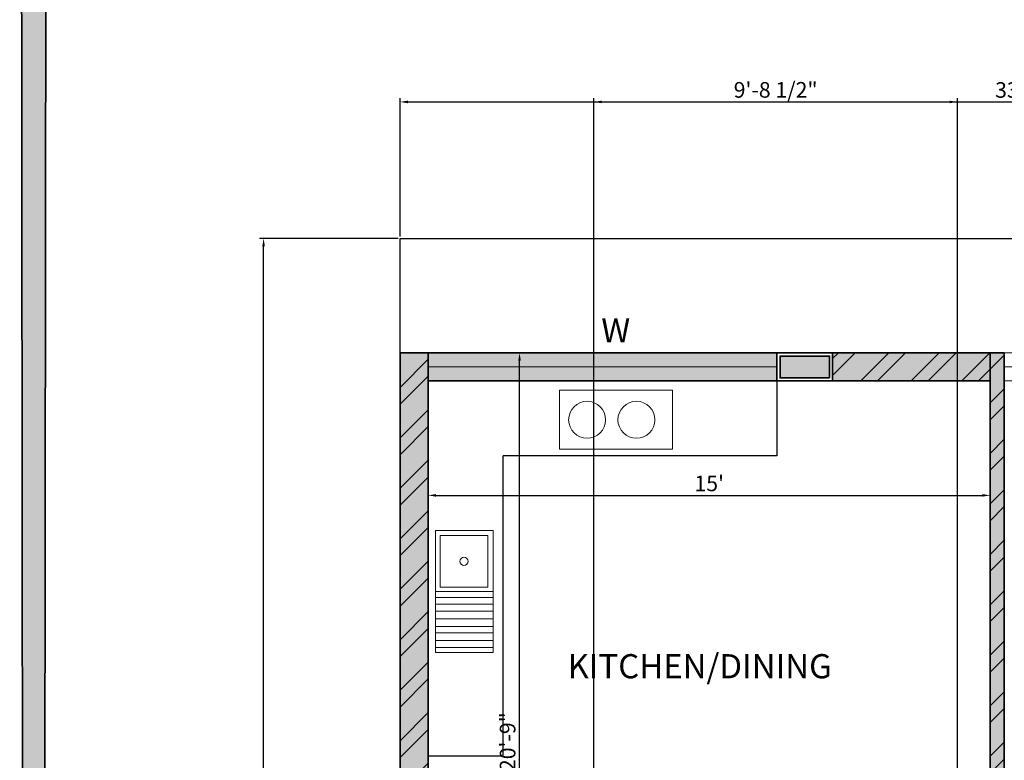
# Model space of a CAD drawing. Units: inches. Extents: x 1804 to 3296, y 909 to 2477.
# Tile 12 of 31: x 1804 to 2119, y 1663 to 1900. Entities that reach past the tile are written whole.
import ezdxf

# ---------------------------------------------------------------- set-up
doc = ezdxf.new("R2010")
doc.units = ezdxf.units.IN
for name, color, linetype, lineweight in [('A-ANNO-DIMS', 2, 'Continuous', 18), ('A-ANNO-TTLB', 156, 'Continuous', 35), ('A-AREA-IDEN', 190, 'Continuous', 18), ('A-EQPM', 9, 'Continuous', 18), ('A-FLOR-CASE', 100, 'Continuous', 25), ('A-FLOR-FIXT', 9, 'Continuous', 18), ('A-WALL-PATT', 10, 'Continuous', 13), ('C-PROP', 7, 'Continuous', 25), ('TEXT', 190, 'Continuous', 18), ('WALL', 10, 'Continuous', 35), ('WIND', 130, 'Continuous', 18)]:
    doc.layers.add(name, color=color, linetype=linetype, lineweight=lineweight)
doc.styles.get("Standard").update_dxf_attribs({"font": 'arial.ttf'})
doc.dimstyles.new('ISO-25', dxfattribs={"dimtxt": 5, "dimasz": 2.5, "dimexe": 1.25, "dimexo": 0.625, "dimtad": 1, "dimdec": 0, "dimlunit": 4, "dimtxsty": 'Standard', "dimcen": 2.5, "dimadec": 0, "dimazin": 0, "dimtfac": 1, "dimtdec": 0, "dimtmove": 0, "dimatfit": 3, "dimfxl": 1, "dimarcsym": 0})
pattern_1 = [(45, (0, 196.207), (-8.08223, 8.08223), []), (45, (5.388, 196.207), (-8.08223, 8.08223), [])]

# ---------------------------------------------------------------- blocks, each defined once
blk = doc.blocks.new('*D8')
at = {"layer": 'A-ANNO-DIMS', "color": 0, "lineweight": -2, "transparency": 16777216}
for p, q in [((1934.58, 1792.75), (1934.58, 1746.51)), ((2114.58, 1792.75), (2114.58, 1746.51)), ((1937.08, 1747.76), (2112.08, 1747.76))]:
    blk.add_line(p, q, dxfattribs=at)
at = {"layer": 'A-ANNO-DIMS', "color": 0, "lineweight": 100, "transparency": 16777216}
for points in [[(1937.08, 1748.17), (1937.08, 1747.34), (1934.58, 1747.76)], [(2112.08, 1748.17), (2112.08, 1747.34), (2114.58, 1747.76)]]:
    blk.add_solid(points, dxfattribs=at)
at = {"layer": 'Defpoints', "color": 0, "lineweight": 100, "transparency": 16777216}
for p in [(1934.58, 1793.38), (2114.58, 1793.38), (2114.58, 1747.76)]:
    blk.add_point(p, dxfattribs=at)
at = {"layer": 'A-ANNO-DIMS', "color": 0, "transparency": 16777216, "insert": (2024.58, 1750.93), "char_height": 5, "attachment_point": 5}
blk.add_mtext("15'", dxfattribs=at)
blk = doc.blocks.new('*D9')
at = {"layer": 'A-ANNO-DIMS', "color": 0, "lineweight": -2, "transparency": 16777216}
for p, q in [((1935.21, 1793.38), (1965.1, 1793.38)), ((1963.85, 1546.88), (1963.85, 1790.88)), ((1935.21, 1544.38), (1965.1, 1544.38))]:
    blk.add_line(p, q, dxfattribs=at)
at = {"layer": 'A-ANNO-DIMS', "color": 0, "lineweight": 100, "transparency": 16777216}
for points in [[(1963.44, 1790.88), (1964.27, 1790.88), (1963.85, 1793.38)], [(1963.44, 1546.88), (1964.27, 1546.88), (1963.85, 1544.38)]]:
    blk.add_solid(points, dxfattribs=at)
at = {"layer": 'Defpoints', "color": 0, "lineweight": 100, "transparency": 16777216}
for p in [(1934.58, 1793.38), (1963.85, 1793.38), (1934.58, 1544.38)]:
    blk.add_point(p, dxfattribs=at)
at = {"layer": 'A-ANNO-DIMS', "color": 0, "transparency": 16777216, "insert": (1960.67, 1668.88), "char_height": 5, "attachment_point": 5, "rotation": 90}
blk.add_mtext('20\'-9"', dxfattribs=at)
blk = doc.blocks.new('WINDOW-PLAN-112IN')
blk.add_line((0, 4.5), (111.7, 4.5))
blk.add_lwpolyline([(0, 0), (111.7, 0), (111.7, 9), (0, 9)], close=True)
blk = doc.blocks.new('*D51')
at = {"layer": 'A-ANNO-DIMS', "color": 0, "lineweight": -2, "transparency": 16777216}
for p, q in [((1925.58, 1830.66), (1925.58, 1874.99)), ((1928.08, 1873.74), (2323.04, 1873.74)), ((2325.54, 1830.66), (2325.54, 1874.99))]:
    blk.add_line(p, q, dxfattribs=at)
at = {"layer": 'A-ANNO-DIMS', "color": 0, "lineweight": 100, "transparency": 16777216}
for points in [[(1928.08, 1874.15), (1928.08, 1873.32), (1925.58, 1873.74)], [(2323.04, 1874.15), (2323.04, 1873.32), (2325.54, 1873.74)]]:
    blk.add_solid(points, dxfattribs=at)
at = {"layer": 'Defpoints', "color": 0, "lineweight": 100, "transparency": 16777216}
for p in [(2325.54, 1873.74), (1925.58, 1830.04), (2325.54, 1830.04)]:
    blk.add_point(p, dxfattribs=at)
at = {"layer": 'A-ANNO-DIMS', "color": 0, "transparency": 16777216, "insert": (2125.56, 1876.92), "char_height": 5, "attachment_point": 5}
blk.add_mtext('33\'-4"', dxfattribs=at)
blk = doc.blocks.new('*D52')
at = {"layer": 'A-ANNO-DIMS', "color": 0, "lineweight": -2, "transparency": 16777216}
for p, q in [((1924.96, 1830.04), (1880.63, 1830.04)), ((1881.88, 1065.27), (1881.88, 1827.54)), ((1924.96, 1062.77), (1880.63, 1062.77))]:
    blk.add_line(p, q, dxfattribs=at)
at = {"layer": 'A-ANNO-DIMS', "color": 0, "lineweight": 100, "transparency": 16777216}
for points in [[(1881.47, 1827.54), (1882.3, 1827.54), (1881.88, 1830.04)], [(1881.47, 1065.27), (1882.3, 1065.27), (1881.88, 1062.77)]]:
    blk.add_solid(points, dxfattribs=at)
at = {"layer": 'Defpoints', "color": 0, "lineweight": 100, "transparency": 16777216}
for p in [(1881.88, 1830.04), (1925.58, 1830.04), (1925.58, 1062.77)]:
    blk.add_point(p, dxfattribs=at)
at = {"layer": 'A-ANNO-DIMS', "color": 0, "transparency": 16777216, "insert": (1878.67, 1446.4), "char_height": 5, "attachment_point": 5, "rotation": 90}
blk.add_mtext('63\'-11 1/2"', dxfattribs=at)
blk = doc.blocks.new('*D62')
at = {"layer": 'A-ANNO-DIMS', "color": 0, "lineweight": -2, "transparency": 16777216}
for p, q in [((1987.63, 1501.57), (1987.63, 1874.99)), ((1990.13, 1873.74), (2101.57, 1873.74)), ((2104.07, 1501.57), (2104.07, 1874.99))]:
    blk.add_line(p, q, dxfattribs=at)
at = {"layer": 'A-ANNO-DIMS', "color": 0, "lineweight": 100, "transparency": 16777216}
for points in [[(1990.13, 1874.15), (1990.13, 1873.32), (1987.63, 1873.74)], [(2101.57, 1874.15), (2101.57, 1873.32), (2104.07, 1873.74)]]:
    blk.add_solid(points, dxfattribs=at)
at = {"layer": 'Defpoints', "color": 0, "lineweight": 100, "transparency": 16777216}
for p in [(2104.07, 1873.74), (1987.63, 1500.95), (2104.07, 1500.95)]:
    blk.add_point(p, dxfattribs=at)
at = {"layer": 'A-ANNO-DIMS', "color": 0, "transparency": 16777216, "insert": (2045.85, 1876.95), "char_height": 5, "attachment_point": 5}
blk.add_mtext('9\'-8 1/2"', dxfattribs=at)

msp = doc.modelspace()

# ---------------------------------------------------------------- hatches: boundary and pattern name
at = {"layer": 'A-ANNO-TTLB'}
h = msp.add_hatch(color=256, dxfattribs=at)
h.dxf.hatch_style = 1
h.paths.add_polyline_path([(3294.53, 2476.54), (1803.79, 2476.54), (1805.43, 909.47), (3296.17, 909.47)])
h.paths.add_polyline_path([(1811, 914.33), (1812.79, 2467.54), (3285.53, 2467.54), (3283.74, 914.33)], flags=16)
h.paths.add_polyline_path([(1925.58, 1062.77), (1925.58, 1138.07), (1925.58, 1539.88), (1925.58, 1793.38), (1925.58, 1830.04), (2325.54, 1830.04), (2325.54, 1793.38), (2325.54, 1586.42), (2325.54, 1138.07), (2325.54, 1062.77)], flags=0)
h.paths.add_polyline_path([(1997.22, 1029.4), (2008.85, 1037.96), (2008.85, 1020.84)], flags=0)
h.paths.add_polyline_path([(1934.58, 1138.07), (1934.58, 1147.07), (2078.77, 1147.07), (2078.77, 1138.07), (2060.94, 1138.07)], flags=0)
h.paths.add_polyline_path([(1944.35, 1138.07), (1944.35, 1147.07), (2056.05, 1147.07), (2056.05, 1138.07)], flags=0)
h.paths.add_polyline_path([(2222.24, 1037.96), (2233.87, 1029.4), (2222.24, 1020.84)], flags=0)
h.paths.add_polyline_path([(2061.94, 1139.07), (2061.94, 1146.07), (2077.77, 1146.07), (2077.77, 1139.07)], flags=0)
h.paths.add_polyline_path([(2149.58, 1138.07), (2149.58, 1269.44), (2158.58, 1269.44), (2158.58, 1326.69), (2149.58, 1326.69), (2149.58, 1340.94), (2139.6, 1340.94), (2139.6, 1434.25), (2149.58, 1434.25), (2149.58, 1447.36), (2158.58, 1447.36), (2158.58, 1423.87), (2158.58, 1408.06), (2198.46, 1408.06), (2198.46, 1412.56), (2282.65, 1412.56), (2282.65, 1465.94), (2316.54, 1465.94), (2316.54, 1590.92), (2192.86, 1590.92), (2192.86, 1595.3), (2291.17, 1595.3), (2291.17, 1590.92), (2316.54, 1590.92), (2316.54, 1784.38), (2300.24, 1784.38), (2300.24, 1757.47), (2268, 1757.47), (2268, 1681.04), (2180.87, 1681.04), (2180.87, 1757.47), (2148.63, 1757.47), (2148.63, 1784.38), (2119.08, 1784.38), (2119.08, 1585.58), (2114.58, 1585.58), (2114.58, 1784.38), (2064.11, 1784.38), (2046.28, 1784.38), (2046.28, 1760.38), (1958.58, 1760.38), (1958.58, 1664.38), (1934.58, 1664.38), (1934.58, 1784.38), (1934.58, 1793.38), (2046.28, 1793.38), (2064.11, 1793.38), (2119.08, 1793.38), (2230.78, 1793.38), (2230.78, 1784.38), (2268, 1784.38), (2300.24, 1784.38), (2316.54, 1784.38), (2316.54, 1590.92), (2316.54, 1373.73), (2316.54, 1138.07)], flags=0)
h.paths.add_polyline_path([(2209.19, 1166.63), (2209.19, 1175.63), (2158.58, 1175.63), (2209.19, 1223.63), (2209.19, 1231.63), (2183.88, 1231.63), (2183.88, 1301.66), (2242.59, 1301.66), (2242.59, 1326.69), (2316.54, 1326.69), (2272.59, 1271.63), (2272.59, 1223.63), (2316.54, 1175.63), (2272.59, 1175.63), (2272.59, 1166.63)], flags=0)
h.paths.add_polyline_path([(1947.77, 1345.22), (1947.77, 1457.48), (1991.2, 1457.48), (1991.2, 1451.7), (1991.2, 1352.18), (1991.2, 1345.22)], flags=0)
h.paths.add_polyline_path([(2209.19, 1271.63), (2262.59, 1271.63), (2262.59, 1311.85), (2272.59, 1301.66), (2272.59, 1271.63), (2269.92, 1269.63), (2270.59, 1269.63), (2270.59, 1225.63), (2211.19, 1225.63), (2211.19, 1269.63), (2211.86, 1269.63)], flags=0)
h.paths.add_polyline_path([(2000.34, 1378.21), (2000.34, 1429.71), (2025.22, 1429.71), (2025.22, 1378.21)], flags=0)
h.paths.add_polyline_path([(2001.34, 1379.21), (2001.34, 1428.71), (2024.22, 1428.71), (2024.22, 1379.21)], flags=0)
h.paths.add_polyline_path([(2012.34, 1390.21), (2012.34, 1417.71), (2013.22, 1417.71), (2013.22, 1390.21)], flags=0)
h.paths.add_polyline_path([(2237.56, 1331.19), (2237.56, 1340.18), (2238.62, 1340.18), (2238.62, 1386.84), (2241.04, 1386.84), (2242.06, 1386.84), (2242.06, 1408.06), (2316.54, 1331.19)], flags=0)
h.paths.add_polyline_path([(1953.73, 1464.35), (1953.73, 1498.59), (1981.74, 1498.59), (1981.74, 1464.35)], flags=0)
h.paths.add_polyline_path([(1987.63, 1462.08), (1987.63, 1500.95), (2104.07, 1500.95), (2104.07, 1462.08), (2099.27, 1462.08), (1993.6, 1462.08)], flags=0)
h.paths.add_polyline_path([(1956.06, 1481.47, -1), (1979.41, 1481.47, -1)], flags=0)
edge = h.paths.add_edge_path(flags=0)
edge.add_ellipse((2299.53, 1438.37), major_axis=(0.31, 21.36), ratio=0.670333, start_angle=0, end_angle=360)
h.paths.add_polyline_path([(2297.39, 1438.37, -1), (2301.67, 1438.37, -1)], flags=0)
h.paths.add_polyline_path([(2591.54, 1163.23), (2591.54, 1179.38), (2591.54, 1379.68), (2591.54, 1395.84), (2734.5, 1395.84), (2734.5, 1379.68), (2734.5, 1179.38), (2734.5, 1163.23)], flags=0)
h.paths.add_polyline_path([(2592.54, 1164.23), (2592.54, 1166.23), (2733.5, 1166.23), (2733.5, 1164.23)], flags=0)
h.paths.add_polyline_path([(2592.54, 1180.38), (2592.54, 1378.68), (2733.5, 1378.68), (2733.5, 1180.38)], flags=0)
h.paths.add_polyline_path([(2593.54, 1181.38), (2593.54, 1377.68), (2732.5, 1377.68), (2732.5, 1181.38)], flags=0)
h.paths.add_polyline_path([(2594.54, 1182.38), (2594.54, 1376.68), (2731.5, 1376.68), (2731.5, 1182.38)], flags=0)
h.paths.add_polyline_path([(1936.95, 1697.46), (1936.95, 1736.46), (1955.41, 1736.46), (1955.41, 1697.46)], flags=0)
h.paths.add_polyline_path([(1938.48, 1718.36), (1938.48, 1734.92), (1953.65, 1734.92), (1953.65, 1718.36)], flags=0)
h.paths.add_polyline_path([(1944.75, 1726.64, -1), (1947.37, 1726.64, -1)], flags=0)
h.paths.add_polyline_path([(2592.54, 1394.84), (2733.5, 1394.84), (2733.5, 1392.84), (2592.54, 1392.84)], flags=0)
h.paths.add_polyline_path([(1976.61, 1762.5), (1976.61, 1781.44), (2012.79, 1781.44), (2012.79, 1762.5)], flags=0)
h.paths.add_polyline_path([(1979.57, 1771.97, -1), (1991.39, 1771.97, -1)], flags=0)
h.paths.add_polyline_path([(1995.36, 1771.97, -1), (2007.18, 1771.97, -1)], flags=0)
h.paths.add_polyline_path([(2251.51, 1744.53), (2268, 1730.05), (2251.51, 1730.05)], flags=0)
h.paths.add_polyline_path([(2047.28, 1785.38), (2047.28, 1792.38), (2063.11, 1792.38), (2063.11, 1785.38)], flags=0)
h.paths.add_polyline_path([(2155.08, 1770.92, -1), (2174.42, 1770.92, -1)], flags=0)
h.paths.add_polyline_path([(2188.59, 1758.27), (2188.59, 1772.81), (2222.3, 1772.81), (2222.3, 1758.27)], flags=0)
h.paths.add_polyline_path([(2223.97, 1758.27), (2223.97, 1772.81), (2257.68, 1772.81), (2257.68, 1758.27)], flags=0)
h.paths.add_polyline_path([(2274.45, 1770.92, -1), (2293.8, 1770.92, -1)], flags=0)
h.paths.add_polyline_path([(2591.54, 1582.09), (2591.54, 1782.39), (2734.5, 1782.39), (2734.5, 1582.09)], flags=0)
h.paths.add_polyline_path([(2592.54, 1583.09), (2592.54, 1781.39), (2733.5, 1781.39), (2733.5, 1583.09)], flags=0)
h.paths.add_polyline_path([(2593.54, 1584.09), (2593.54, 1780.39), (2732.5, 1780.39), (2732.5, 1584.09)], flags=0)
h.paths.add_polyline_path([(2594.54, 1585.09), (2594.54, 1779.39), (2731.5, 1779.39), (2731.5, 1585.09)], flags=0)
h.paths.add_polyline_path([(1922.17, 1978.79), (1922.17, 2295.08), (1922.17, 2296.08), (2115.67, 2296.08), (2115.67, 2384.31), (2115.67, 2385.31), (2322.12, 2385.31), (2323.12, 2385.31), (2323.12, 1979.79), (2323.12, 1978.79), (1923.17, 1978.79)], flags=0)
h.paths.add_polyline_path([(1922.17, 1978.79), (1922.17, 2051.31), (1922.17, 2214.86), (1922.17, 2296.08), (2115.67, 2296.08), (2115.67, 2385.31), (2323.12, 2385.31), (2323.12, 2280.42), (2323.12, 1978.79), (2115.67, 1978.79)], flags=0)
h.paths.add_polyline_path([(1923.17, 1979.79), (1923.17, 2050.31), (2115.67, 2050.31), (2115.67, 2051.31), (1923.17, 2051.31), (1923.17, 2213.86), (1923.17, 2214.86), (1923.17, 2295.08), (1990.02, 2295.08), (1990.02, 2214.86), (1991.02, 2214.86), (1991.02, 2295.08), (2115.67, 2295.08), (2115.67, 1979.79), (2116.67, 1979.79), (2116.67, 2304.18), (2116.67, 2384.31), (2322.12, 2384.31), (2322.12, 2280.42), (2322.12, 1979.79), (2115.67, 1979.79)], flags=0)
h.paths.add_polyline_path([(2972.46, 1192.5), (2972.46, 1196.92), (2995.47, 1196.92), (2995.47, 1255.47), (2995.09, 1255.47), (2987.42, 1249.39), (2980.08, 1255.47), (2978.05, 1255.47), (2978.05, 1257.24), (2995.47, 1257.24), (2995.47, 1261.58), (3015.37, 1261.58), (3015.37, 1333.28), (3015.37, 1414.4), (3032.82, 1414.4), (3032.82, 1333.28), (3032.82, 1261.58), (3052.66, 1261.58), (3052.66, 1255.47), (3079.86, 1255.47), (3078.72, 1254.57), (3081.47, 1252.29), (3078.56, 1249.99), (3075.81, 1252.26), (3072.57, 1249.69), (3070.36, 1251.52), (3067.67, 1249.39), (3060.34, 1255.47), (3052.66, 1255.47), (3052.66, 1196.92), (3054.58, 1196.92), (3074, 1196.92), (3074, 1192.5), (3052.66, 1192.5), (2995.47, 1192.5)], flags=0)
h.paths.add_polyline_path([(2490.75, 1979.27), (2490.75, 1980.27), (2596.87, 1980.27), (2596.87, 2051.8), (2596.87, 2052.8), (2596.87, 2216.35), (2596.87, 2297.57), (2717.32, 2297.57), (2710.57, 2305.62), (2724.07, 2305.62), (2717.32, 2297.57), (2782.37, 2297.57), (2782.37, 2395.8), (3006.82, 2395.8), (3006.82, 1981.27), (3093.73, 1981.27), (3093.73, 1980.27), (3047.51, 1980.27), (3046.37, 1979.37), (3049.11, 1977.1), (3046.2, 1974.79), (3043.46, 1977.07), (3040.21, 1974.49), (3038, 1976.32), (3035.32, 1974.2), (3027.98, 1980.27), (2871.83, 1980.27), (2871.83, 1981.27), (2791.37, 1981.27), (2791.37, 2050.8), (2597.87, 2050.8), (2597.87, 1980.27), (2597.87, 1979.27), (2546.27, 1979.27), (2545.12, 1978.37), (2547.87, 1976.1), (2544.96, 1973.79), (2542.22, 1976.07), (2538.97, 1973.49), (2536.76, 1975.32), (2534.07, 1973.2), (2526.74, 1979.27)], flags=0)
h.paths.add_polyline_path([(2597.87, 2051.8), (2606.87, 2051.8), (2606.87, 2258.39), (2597.87, 2258.39), (2597.87, 2296.57), (2606.87, 2296.57), (2606.87, 2262.39), (2782.37, 2262.39), (2782.37, 2296.57), (2790.37, 2296.57), (2790.37, 2262.39), (2791.37, 2262.39), (2791.37, 2305.67), (2791.37, 2385.8), (2996.82, 2385.8), (2996.82, 2339.85), (3006.82, 2339.85), (3006.82, 2250.12), (2997.82, 2250.12), (2997.82, 1981.27), (2996.82, 1981.27), (2872.83, 1981.27), (2872.83, 1991.8), (2871.83, 1991.8), (2871.83, 2050.8), (2790.37, 2050.8), (2597.87, 2050.8)], flags=0)
h.paths.add_polyline_path([(2179.93, 2153.92), (2179.93, 2353.97), (2259.98, 2353.97), (2259.98, 2153.92)], flags=0)
h.paths.add_polyline_path([(2180.93, 2154.92), (2180.93, 2352.97), (2258.98, 2352.97), (2258.98, 2154.92)], flags=0)
h.paths.add_polyline_path([(2960.87, 1608.49), (2960.87, 1753.62), (3070.9, 1753.62), (3070.9, 1608.49)], flags=0)
h.paths.add_polyline_path([(2961.87, 1609.49), (2961.87, 1752.62), (3069.9, 1752.62), (3069.9, 1609.49)], flags=0)
h.paths.add_polyline_path([(2962.87, 1610.49), (2962.87, 1751.62), (3068.9, 1751.62), (3068.9, 1610.49)], flags=0)
h.paths.add_polyline_path([(2963.87, 1611.49), (2963.87, 1750.62), (3067.9, 1750.62), (3067.9, 1611.49)], flags=0)
h.paths.add_polyline_path([(2782.37, 2051.8), (2782.37, 2216.32), (2791.37, 2216.32), (2791.37, 2051.8), (2872.83, 2051.8), (2872.83, 2068.56), (2884.67, 2068.56), (2884.67, 2085.33), (2896.51, 2085.33), (2896.51, 2102.09), (2908.36, 2102.09), (2908.36, 2118.85), (2920.2, 2118.85), (2920.2, 2135.62), (2932.05, 2135.62), (2932.05, 2145.3), (2925.08, 2145.3), (2925.08, 2203.2), (2996.82, 2203.2), (2996.82, 2145.3), (2953.82, 2145.3), (2872.83, 2051.8), (2790.37, 2051.8)], flags=0)
h.paths.add_polyline_path([(2717.32, 2238.65), (2710.57, 2246.7), (2724.07, 2246.7)], flags=0)
h.paths.add_polyline_path([(2003.09, 1122.79), (2017.16, 1122.79), (2017.16, 1138.74), (2003.09, 1138.74)], flags=8)
h.paths.add_polyline_path([(2174.76, 1792.72), (2188.83, 1792.72), (2188.83, 1808.66), (2174.76, 1808.66)], flags=8)
h.paths.add_polyline_path([(1987.95, 1792.51), (2002.02, 1792.51), (2002.02, 1808.45), (1987.95, 1808.45)], flags=8)
h.paths.add_polyline_path([(2148.79, 1289.26), (2160.46, 1289.26), (2160.46, 1305.2), (2148.79, 1305.2)], flags=8)
h.paths.add_polyline_path([(2115.36, 1133.57), (2127.04, 1133.57), (2127.04, 1149.51), (2115.36, 1149.51)], flags=8)
h.paths.add_polyline_path([(2237.58, 1421.48), (2249.25, 1421.48), (2249.25, 1437.43), (2237.58, 1437.43)], flags=8)
h.paths.add_polyline_path([(2134.99, 1584.32), (2146.66, 1584.32), (2146.66, 1600.26), (2134.99, 1600.26)], flags=8)
h.paths.add_polyline_path([(2101.95, 1557.31), (2113.62, 1557.31), (2113.62, 1573.25), (2101.95, 1573.25)], flags=8)
h.paths.add_polyline_path([(2937.85, 1156.77), (3120.41, 1156.77), (3120.41, 1185.72), (2937.85, 1185.72)], flags=8)
h.paths.add_polyline_path([(2980.71, 1786.71), (3050.06, 1786.71), (3050.06, 1802.66), (2980.71, 1802.66)], flags=8)
h.paths.add_polyline_path([(2869.28, 1661.96), (2938.62, 1661.96), (2938.62, 1690.8), (2869.28, 1690.8)], flags=8)
h.paths.add_polyline_path([(3092.27, 1674.86), (3161.62, 1674.86), (3161.62, 1690.8), (3092.27, 1690.8)], flags=8)
h.paths.add_polyline_path([(2980.71, 1674.86), (3050.06, 1674.86), (3050.06, 1690.8), (2980.71, 1690.8)], flags=8)
h.paths.add_polyline_path([(2649.07, 1678.23), (2674.53, 1678.23), (2674.53, 1714.76), (2649.07, 1714.76)], flags=8)
h.paths.add_polyline_path([(2530.84, 1981.63), (2549.13, 1981.63), (2549.13, 1997.57), (2530.84, 1997.57)], flags=8)
h.paths.add_polyline_path([(3031.29, 1981.77), (3049.58, 1981.77), (3049.58, 1997.71), (3031.29, 1997.71)], flags=8)
h.paths.add_polyline_path([(2715.38, 1911.9), (2851.54, 1911.9), (2851.54, 1940.85), (2715.38, 1940.85)], flags=8)
h.paths.add_polyline_path([(2015.23, 1927.36), (2205.42, 1927.36), (2205.42, 1956.3), (2015.23, 1956.3)], flags=8)
h.paths.add_polyline_path([(2671.84, 2057.84), (2702.75, 2057.84), (2702.75, 2073.79), (2671.84, 2073.79)], flags=8)
h.paths.add_polyline_path([(2678.5, 2316.52), (2765.26, 2316.52), (2765.26, 2332.46), (2678.5, 2332.46)], flags=8)
h.paths.add_polyline_path([(2678.48, 2271.96), (2736.41, 2271.96), (2736.41, 2287.9), (2678.48, 2287.9)], flags=8)
h.paths.add_polyline_path([(2019.2, 972.79), (2243.21, 972.79), (2243.21, 1001.74), (2019.2, 1001.74)], flags=8)
h.paths.add_polyline_path([(2097.06, 1021.56), (2132.16, 1021.56), (2132.16, 1037.51), (2097.06, 1037.51)], flags=8)
h.paths.add_polyline_path([(2182.47, 1360.48), (2207.35, 1360.48), (2207.35, 1376.42), (2182.47, 1376.42)], flags=8)
h.paths.add_polyline_path([(2261.12, 1361.77), (2295.01, 1361.77), (2295.01, 1377.71), (2261.12, 1377.71)], flags=8)
h.paths.add_polyline_path([(2245.75, 1511.51), (2278.44, 1511.51), (2278.44, 1527.46), (2245.75, 1527.46)], flags=8)
h.paths.add_polyline_path([(1991.16, 1296.29), (2060.51, 1296.29), (2060.51, 1312.23), (1991.16, 1312.23)], flags=8)
h.paths.add_polyline_path([(2187, 1651.35), (2246.71, 1651.35), (2246.71, 1667.29), (2187, 1667.29)], flags=8)
h.paths.add_polyline_path([(1976.49, 1684.81), (2068.63, 1684.81), (2068.63, 1700.76), (1976.49, 1700.76)], flags=8)
at = {"layer": 'A-WALL-PATT'}
h = msp.add_hatch(color=256, dxfattribs=at)
h.dxf.hatch_style = 1
h.paths.add_polyline_path([(2119.08, 1544.38), (1925.58, 1544.38), (1925.58, 1539.88), (2119.08, 1539.88)])
h.paths.add_polyline_path([(2119.08, 1545.58), (2114.58, 1545.58), (2114.58, 1544.38), (2119.08, 1544.38)])
h.paths.add_polyline_path([(1965.87, 1658.79), (1965.87, 1679.09), (1955.57, 1679.09), (1955.57, 1658.79)], flags=9)
h.paths.add_polyline_path([(2293.18, 1677.29), (2293.18, 1697.58), (2282.88, 1697.58), (2282.88, 1677.29)], flags=9)
h.paths.add_polyline_path([(2271.13, 1545.23), (2287.53, 1545.23), (2287.53, 1555.53), (2271.13, 1555.53)], flags=9)
h.paths.add_polyline_path([(2303.26, 1488.52), (2303.26, 1508.82), (2292.95, 1508.82), (2292.95, 1488.52)], flags=9)
h.paths.add_polyline_path([(2271.13, 1393.15), (2287.53, 1393.15), (2287.53, 1403.45), (2271.13, 1403.45)], flags=9)
h.paths.add_polyline_path([(2306.48, 1361.45), (2306.48, 1377.86), (2296.18, 1377.86), (2296.18, 1361.45)], flags=9)
h.paths.add_polyline_path([(2174.54, 1361.45), (2174.54, 1377.86), (2164.23, 1377.86), (2164.23, 1361.45)], flags=9)
h.paths.add_polyline_path([(1968.21, 1333.34), (1968.21, 1353.64), (1957.91, 1353.64), (1957.91, 1333.34)], flags=9)
h.paths.add_polyline_path([(2003.09, 1122.79), (2017.16, 1122.79), (2017.16, 1138.74), (2003.09, 1138.74)], flags=9)
h.paths.add_polyline_path([(2174.76, 1792.72), (2188.83, 1792.72), (2188.83, 1808.66), (2174.76, 1808.66)], flags=9)
h.paths.add_polyline_path([(1987.95, 1792.51), (2002.02, 1792.51), (2002.02, 1808.45), (1987.95, 1808.45)], flags=9)
h.paths.add_polyline_path([(2148.79, 1289.26), (2160.46, 1289.26), (2160.46, 1305.2), (2148.79, 1305.2)], flags=9)
h.paths.add_polyline_path([(2115.36, 1133.57), (2127.04, 1133.57), (2127.04, 1149.51), (2115.36, 1149.51)], flags=9)
h.paths.add_polyline_path([(2237.58, 1421.48), (2249.25, 1421.48), (2249.25, 1437.43), (2237.58, 1437.43)], flags=9)
h.paths.add_polyline_path([(2134.99, 1584.32), (2146.66, 1584.32), (2146.66, 1600.26), (2134.99, 1600.26)], flags=9)
h.paths.add_polyline_path([(2101.95, 1557.31), (2113.62, 1557.31), (2113.62, 1573.25), (2101.95, 1573.25)], flags=9)
h.paths.add_polyline_path([(2937.85, 1156.77), (3120.41, 1156.77), (3120.41, 1185.72), (2937.85, 1185.72)], flags=9)
h.paths.add_polyline_path([(2980.71, 1786.71), (3050.06, 1786.71), (3050.06, 1802.66), (2980.71, 1802.66)], flags=9)
h.paths.add_polyline_path([(2869.28, 1661.96), (2938.62, 1661.96), (2938.62, 1690.8), (2869.28, 1690.8)], flags=9)
h.paths.add_polyline_path([(3092.27, 1674.86), (3161.62, 1674.86), (3161.62, 1690.8), (3092.27, 1690.8)], flags=9)
h.paths.add_polyline_path([(2980.71, 1674.86), (3050.06, 1674.86), (3050.06, 1690.8), (2980.71, 1690.8)], flags=9)
h.paths.add_polyline_path([(2649.07, 1678.23), (2674.53, 1678.23), (2674.53, 1714.76), (2649.07, 1714.76)], flags=9)
h.paths.add_polyline_path([(2530.84, 1981.63), (2549.13, 1981.63), (2549.13, 1997.57), (2530.84, 1997.57)], flags=9)
h.paths.add_polyline_path([(3031.29, 1981.77), (3049.58, 1981.77), (3049.58, 1997.71), (3031.29, 1997.71)], flags=9)
h.paths.add_polyline_path([(2715.38, 1911.9), (2851.54, 1911.9), (2851.54, 1940.85), (2715.38, 1940.85)], flags=9)
h.paths.add_polyline_path([(2015.23, 1927.36), (2205.42, 1927.36), (2205.42, 1956.3), (2015.23, 1956.3)], flags=9)
h.paths.add_polyline_path([(2671.84, 2057.84), (2702.75, 2057.84), (2702.75, 2073.79), (2671.84, 2073.79)], flags=9)
h.paths.add_polyline_path([(2678.5, 2316.52), (2765.26, 2316.52), (2765.26, 2332.46), (2678.5, 2332.46)], flags=9)
h.paths.add_polyline_path([(2678.48, 2271.96), (2736.41, 2271.96), (2736.41, 2287.9), (2678.48, 2287.9)], flags=9)
h.paths.add_polyline_path([(2019.2, 972.79), (2243.21, 972.79), (2243.21, 1001.74), (2019.2, 1001.74)], flags=9)
h.paths.add_polyline_path([(2097.06, 1021.56), (2132.16, 1021.56), (2132.16, 1037.51), (2097.06, 1037.51)], flags=9)
h.paths.add_polyline_path([(2182.47, 1360.48), (2207.35, 1360.48), (2207.35, 1376.42), (2182.47, 1376.42)], flags=9)
h.paths.add_polyline_path([(2261.12, 1361.77), (2295.01, 1361.77), (2295.01, 1377.71), (2261.12, 1377.71)], flags=9)
h.paths.add_polyline_path([(2245.75, 1511.51), (2278.44, 1511.51), (2278.44, 1527.46), (2245.75, 1527.46)], flags=9)
h.paths.add_polyline_path([(1991.16, 1296.29), (2060.51, 1296.29), (2060.51, 1312.23), (1991.16, 1312.23)], flags=9)
h.paths.add_polyline_path([(2187, 1651.35), (2246.71, 1651.35), (2246.71, 1667.29), (2187, 1667.29)], flags=9)
h.paths.add_polyline_path([(1976.49, 1684.81), (2068.63, 1684.81), (2068.63, 1700.76), (1976.49, 1700.76)], flags=9)
h = msp.add_hatch(color=256, dxfattribs=at)
h.dxf.hatch_style = 1
h.paths.add_polyline_path([(2149.58, 1147.07), (2141.21, 1147.07), (2141.21, 1144.07), (2141.21, 1138.07), (2149.58, 1138.07)])
h.paths.add_polyline_path([(2101.21, 1144.07, -0.01877), (2101.32, 1147.07), (2078.77, 1147.07), (2078.77, 1138.07), (2101.21, 1138.07)])
h.paths.add_polyline_path([(2060.94, 1147.07), (2056.05, 1147.07), (2056.05, 1138.07), (2060.94, 1138.07)])
h.paths.add_polyline_path([(1944.35, 1147.07), (1934.58, 1147.07), (1934.58, 1138.07), (1944.35, 1138.07)])
h.paths.add_polyline_path([(2158.58, 1269.44), (2149.58, 1269.44), (2149.58, 1138.07), (2158.58, 1138.07)])
h.paths.add_polyline_path([(2003.09, 1122.79), (2017.16, 1122.79), (2017.16, 1138.74), (2003.09, 1138.74)], flags=9)
h.paths.add_polyline_path([(2174.76, 1792.72), (2188.83, 1792.72), (2188.83, 1808.66), (2174.76, 1808.66)], flags=9)
h.paths.add_polyline_path([(1987.95, 1792.51), (2002.02, 1792.51), (2002.02, 1808.45), (1987.95, 1808.45)], flags=9)
h.paths.add_polyline_path([(2148.79, 1289.26), (2160.46, 1289.26), (2160.46, 1305.2), (2148.79, 1305.2)], flags=9)
h.paths.add_polyline_path([(2115.36, 1133.57), (2127.04, 1133.57), (2127.04, 1149.51), (2115.36, 1149.51)], flags=9)
h.paths.add_polyline_path([(2237.58, 1421.48), (2249.25, 1421.48), (2249.25, 1437.43), (2237.58, 1437.43)], flags=9)
h.paths.add_polyline_path([(2134.99, 1584.32), (2146.66, 1584.32), (2146.66, 1600.26), (2134.99, 1600.26)], flags=9)
h.paths.add_polyline_path([(2101.95, 1557.31), (2113.62, 1557.31), (2113.62, 1573.25), (2101.95, 1573.25)], flags=9)
h.paths.add_polyline_path([(2937.85, 1156.77), (3120.41, 1156.77), (3120.41, 1185.72), (2937.85, 1185.72)], flags=9)
h.paths.add_polyline_path([(2980.71, 1786.71), (3050.06, 1786.71), (3050.06, 1802.66), (2980.71, 1802.66)], flags=9)
h.paths.add_polyline_path([(2869.28, 1661.96), (2938.62, 1661.96), (2938.62, 1690.8), (2869.28, 1690.8)], flags=9)
h.paths.add_polyline_path([(3092.27, 1674.86), (3161.62, 1674.86), (3161.62, 1690.8), (3092.27, 1690.8)], flags=9)
h.paths.add_polyline_path([(2980.71, 1674.86), (3050.06, 1674.86), (3050.06, 1690.8), (2980.71, 1690.8)], flags=9)
h.paths.add_polyline_path([(2649.07, 1678.23), (2674.53, 1678.23), (2674.53, 1714.76), (2649.07, 1714.76)], flags=9)
h.paths.add_polyline_path([(2530.84, 1981.63), (2549.13, 1981.63), (2549.13, 1997.57), (2530.84, 1997.57)], flags=9)
h.paths.add_polyline_path([(3031.29, 1981.77), (3049.58, 1981.77), (3049.58, 1997.71), (3031.29, 1997.71)], flags=9)
h.paths.add_polyline_path([(2715.38, 1911.9), (2851.54, 1911.9), (2851.54, 1940.85), (2715.38, 1940.85)], flags=9)
h.paths.add_polyline_path([(2015.23, 1927.36), (2205.42, 1927.36), (2205.42, 1956.3), (2015.23, 1956.3)], flags=9)
h.paths.add_polyline_path([(2671.84, 2057.84), (2702.75, 2057.84), (2702.75, 2073.79), (2671.84, 2073.79)], flags=9)
h.paths.add_polyline_path([(2678.5, 2316.52), (2765.26, 2316.52), (2765.26, 2332.46), (2678.5, 2332.46)], flags=9)
h.paths.add_polyline_path([(2678.48, 2271.96), (2736.41, 2271.96), (2736.41, 2287.9), (2678.48, 2287.9)], flags=9)
h.paths.add_polyline_path([(2019.2, 972.79), (2243.21, 972.79), (2243.21, 1001.74), (2019.2, 1001.74)], flags=9)
h.paths.add_polyline_path([(2097.06, 1021.56), (2132.16, 1021.56), (2132.16, 1037.51), (2097.06, 1037.51)], flags=9)
h.paths.add_polyline_path([(2182.47, 1360.48), (2207.35, 1360.48), (2207.35, 1376.42), (2182.47, 1376.42)], flags=9)
h.paths.add_polyline_path([(2261.12, 1361.77), (2295.01, 1361.77), (2295.01, 1377.71), (2261.12, 1377.71)], flags=9)
h.paths.add_polyline_path([(2245.75, 1511.51), (2278.44, 1511.51), (2278.44, 1527.46), (2245.75, 1527.46)], flags=9)
h.paths.add_polyline_path([(1991.16, 1296.29), (2060.51, 1296.29), (2060.51, 1312.23), (1991.16, 1312.23)], flags=9)
h.paths.add_polyline_path([(2187, 1651.35), (2246.71, 1651.35), (2246.71, 1667.29), (2187, 1667.29)], flags=9)
h.paths.add_polyline_path([(1976.49, 1684.81), (2068.63, 1684.81), (2068.63, 1700.76), (1976.49, 1700.76)], flags=9)
h = msp.add_hatch(color=256, dxfattribs=at)
h.dxf.hatch_style = 1
h.paths.add_polyline_path([(2158.58, 1275.49), (2155.29, 1275.49), (2149.58, 1275.49), (2149.58, 1269.44), (2158.58, 1269.44)])
h.paths.add_polyline_path([(2158.58, 1326.69), (2149.58, 1326.69), (2149.58, 1319.33), (2155.29, 1319.33), (2158.58, 1319.33)])
h.paths.add_polyline_path([(2158.58, 1402.2), (2158.58, 1423.87), (2158.58, 1447.36), (2149.58, 1447.36), (2149.58, 1423.87), (2149.58, 1340.94), (2149.58, 1326.69), (2158.58, 1326.69), (2158.58, 1354.23)])
h.paths.add_polyline_path([(1965.87, 1658.79), (1965.87, 1679.09), (1955.57, 1679.09), (1955.57, 1658.79)], flags=9)
h.paths.add_polyline_path([(2293.18, 1677.29), (2293.18, 1697.58), (2282.88, 1697.58), (2282.88, 1677.29)], flags=9)
h.paths.add_polyline_path([(2271.13, 1545.23), (2287.53, 1545.23), (2287.53, 1555.53), (2271.13, 1555.53)], flags=9)
h.paths.add_polyline_path([(2303.26, 1488.52), (2303.26, 1508.82), (2292.95, 1508.82), (2292.95, 1488.52)], flags=9)
h.paths.add_polyline_path([(2271.13, 1393.15), (2287.53, 1393.15), (2287.53, 1403.45), (2271.13, 1403.45)], flags=9)
h.paths.add_polyline_path([(2306.48, 1361.45), (2306.48, 1377.86), (2296.18, 1377.86), (2296.18, 1361.45)], flags=9)
h.paths.add_polyline_path([(2189.9, 1340.62), (2206.31, 1340.62), (2206.31, 1350.92), (2189.9, 1350.92)], flags=9)
h.paths.add_polyline_path([(2174.54, 1361.45), (2174.54, 1377.86), (2164.23, 1377.86), (2164.23, 1361.45)], flags=9)
h.paths.add_polyline_path([(2304.24, 1240.8), (2304.24, 1261.09), (2293.94, 1261.09), (2293.94, 1240.8)], flags=9)
h.paths.add_polyline_path([(2227.19, 1188.73), (2247.49, 1188.73), (2247.49, 1199.03), (2227.19, 1199.03)], flags=9)
h.paths.add_polyline_path([(2181.93, 1144.21), (2181.93, 1160.62), (2171.63, 1160.62), (2171.63, 1144.21)], flags=9)
h.paths.add_polyline_path([(1968.21, 1333.34), (1968.21, 1353.64), (1957.91, 1353.64), (1957.91, 1333.34)], flags=9)
h.paths.add_polyline_path([(2029.78, 1203.53), (2053.95, 1203.53), (2053.95, 1213.83), (2029.78, 1213.83)], flags=9)
h.paths.add_polyline_path([(2576.51, 1671.88), (2576.51, 1692.17), (2566.21, 1692.17), (2566.21, 1671.88)], flags=9)
h.paths.add_polyline_path([(2566.99, 1269.67), (2566.99, 1289.96), (2556.68, 1289.96), (2556.68, 1269.67)], flags=9)
h.paths.add_polyline_path([(2581.85, 1269.17), (2581.85, 1289.46), (2571.54, 1289.46), (2571.54, 1269.17)], flags=9)
h.paths.add_polyline_path([(2650.71, 1409.75), (2674.89, 1409.75), (2674.89, 1420.05), (2650.71, 1420.05)], flags=9)
h.paths.add_polyline_path([(2003.09, 1122.79), (2017.16, 1122.79), (2017.16, 1138.74), (2003.09, 1138.74)], flags=9)
h.paths.add_polyline_path([(2174.76, 1792.72), (2188.83, 1792.72), (2188.83, 1808.66), (2174.76, 1808.66)], flags=9)
h.paths.add_polyline_path([(1987.95, 1792.51), (2002.02, 1792.51), (2002.02, 1808.45), (1987.95, 1808.45)], flags=9)
h.paths.add_polyline_path([(2148.79, 1289.26), (2160.46, 1289.26), (2160.46, 1305.2), (2148.79, 1305.2)], flags=9)
h.paths.add_polyline_path([(2115.36, 1133.57), (2127.04, 1133.57), (2127.04, 1149.51), (2115.36, 1149.51)], flags=9)
h.paths.add_polyline_path([(2237.58, 1421.48), (2249.25, 1421.48), (2249.25, 1437.43), (2237.58, 1437.43)], flags=9)
h.paths.add_polyline_path([(2134.99, 1584.32), (2146.66, 1584.32), (2146.66, 1600.26), (2134.99, 1600.26)], flags=9)
h.paths.add_polyline_path([(2101.95, 1557.31), (2113.62, 1557.31), (2113.62, 1573.25), (2101.95, 1573.25)], flags=9)
h.paths.add_polyline_path([(2937.85, 1156.77), (3120.41, 1156.77), (3120.41, 1185.72), (2937.85, 1185.72)], flags=9)
h.paths.add_polyline_path([(2980.71, 1786.71), (3050.06, 1786.71), (3050.06, 1802.66), (2980.71, 1802.66)], flags=9)
h.paths.add_polyline_path([(2869.28, 1661.96), (2938.62, 1661.96), (2938.62, 1690.8), (2869.28, 1690.8)], flags=9)
h.paths.add_polyline_path([(3092.27, 1674.86), (3161.62, 1674.86), (3161.62, 1690.8), (3092.27, 1690.8)], flags=9)
h.paths.add_polyline_path([(2980.71, 1674.86), (3050.06, 1674.86), (3050.06, 1690.8), (2980.71, 1690.8)], flags=9)
h.paths.add_polyline_path([(2649.07, 1678.23), (2674.53, 1678.23), (2674.53, 1714.76), (2649.07, 1714.76)], flags=9)
h.paths.add_polyline_path([(2530.84, 1981.63), (2549.13, 1981.63), (2549.13, 1997.57), (2530.84, 1997.57)], flags=9)
h.paths.add_polyline_path([(3031.29, 1981.77), (3049.58, 1981.77), (3049.58, 1997.71), (3031.29, 1997.71)], flags=9)
h.paths.add_polyline_path([(2715.38, 1911.9), (2851.54, 1911.9), (2851.54, 1940.85), (2715.38, 1940.85)], flags=9)
h.paths.add_polyline_path([(2015.23, 1927.36), (2205.42, 1927.36), (2205.42, 1956.3), (2015.23, 1956.3)], flags=9)
h.paths.add_polyline_path([(2671.84, 2057.84), (2702.75, 2057.84), (2702.75, 2073.79), (2671.84, 2073.79)], flags=9)
h.paths.add_polyline_path([(2678.5, 2316.52), (2765.26, 2316.52), (2765.26, 2332.46), (2678.5, 2332.46)], flags=9)
h.paths.add_polyline_path([(2678.48, 2271.96), (2736.41, 2271.96), (2736.41, 2287.9), (2678.48, 2287.9)], flags=9)
h.paths.add_polyline_path([(2019.2, 972.79), (2243.21, 972.79), (2243.21, 1001.74), (2019.2, 1001.74)], flags=9)
h.paths.add_polyline_path([(2097.06, 1021.56), (2132.16, 1021.56), (2132.16, 1037.51), (2097.06, 1037.51)], flags=9)
h.paths.add_polyline_path([(2182.47, 1360.48), (2207.35, 1360.48), (2207.35, 1376.42), (2182.47, 1376.42)], flags=9)
h.paths.add_polyline_path([(2261.12, 1361.77), (2295.01, 1361.77), (2295.01, 1377.71), (2261.12, 1377.71)], flags=9)
h.paths.add_polyline_path([(2245.75, 1511.51), (2278.44, 1511.51), (2278.44, 1527.46), (2245.75, 1527.46)], flags=9)
h.paths.add_polyline_path([(1991.16, 1296.29), (2060.51, 1296.29), (2060.51, 1312.23), (1991.16, 1312.23)], flags=9)
h.paths.add_polyline_path([(2187, 1651.35), (2246.71, 1651.35), (2246.71, 1667.29), (2187, 1667.29)], flags=9)
h.paths.add_polyline_path([(1976.49, 1684.81), (2068.63, 1684.81), (2068.63, 1700.76), (1976.49, 1700.76)], flags=9)
h = msp.add_hatch(dxfattribs=at)
h.set_pattern_fill('ANSI32', color=256, scale=1.2)
h.set_pattern_definition(pattern_1)
h.paths.add_polyline_path([(1934.58, 1784.38), (1934.58, 1793.38), (1925.58, 1793.38), (1925.58, 1539.88), (2119.08, 1539.88), (2119.08, 1545.58), (2114.58, 1545.58), (2114.58, 1544.38), (1934.58, 1544.38)])
h.paths.add_polyline_path([(2114.58, 1793.38), (2064.11, 1793.38), (2064.11, 1784.38), (2114.58, 1784.38)], flags=17)
h.paths.add_polyline_path([(2325.54, 1793.38), (2230.78, 1793.38), (2230.78, 1784.38), (2268, 1784.38), (2300.24, 1784.38), (2316.54, 1784.38), (2316.54, 1590.92), (2316.54, 1586.42), (2325.54, 1586.42)])
h.paths.add_polyline_path([(1944.35, 1147.07), (1934.58, 1147.07), (1934.58, 1138.07), (1944.35, 1138.07)])
h.paths.add_polyline_path([(2101.21, 1144.07, -0.01877), (2101.32, 1147.07), (2078.77, 1147.07), (2078.77, 1138.07), (2101.21, 1138.07)])
h.paths.add_polyline_path([(1934.58, 1539.88), (1925.58, 1539.88), (1925.58, 1138.07), (1934.58, 1138.07), (1934.58, 1147.07)])
h.paths.add_polyline_path([(2325.54, 1586.42), (2316.54, 1586.42), (2316.54, 1373.73), (2316.54, 1138.07), (2325.54, 1138.07), (2325.54, 1228.97)])
h.paths.add_polyline_path([(2158.58, 1423.87), (2158.58, 1447.36), (2149.58, 1447.36), (2149.58, 1423.87), (2149.58, 1340.94), (2149.58, 1326.69), (2158.58, 1326.69), (2158.58, 1354.23), (2158.58, 1402.2)])
h.paths.add_polyline_path([(2316.54, 1412.56), (2282.65, 1412.56), (2273.09, 1412.56), (2273.09, 1408.06), (2316.54, 1408.06)])
h.paths.add_polyline_path([(2273.09, 1412.56), (2242.06, 1412.56), (2242.06, 1408.06), (2273.09, 1408.06)])
h.paths.add_polyline_path([(2237.56, 1412.56), (2198.46, 1412.56), (2198.46, 1408.06), (2237.56, 1408.06)])
h.paths.add_polyline_path([(2242.06, 1408.06), (2237.56, 1408.06), (2237.56, 1386.84), (2242.06, 1386.84)])
h.paths.add_polyline_path([(2242.06, 1412.56), (2237.56, 1412.56), (2237.56, 1408.06), (2242.06, 1408.06)])
h.paths.add_polyline_path([(2158.58, 1269.44), (2149.58, 1269.44), (2149.58, 1138.07), (2158.58, 1138.07)])
h.paths.add_polyline_path([(2149.58, 1147.07), (2141.21, 1147.07), (2141.21, 1144.07), (2141.21, 1138.07), (2149.58, 1138.07)])
h.paths.add_polyline_path([(2272.59, 1175.63), (2209.19, 1175.63), (2209.19, 1166.63), (2272.59, 1166.63)])
h.paths.add_polyline_path([(2237.56, 1446.21), (2242.06, 1446.21), (2242.06, 1586.42), (2237.56, 1586.42)])
h.paths.add_polyline_path([(2242.06, 1414.58), (2237.56, 1414.58), (2237.56, 1412.56), (2242.06, 1412.56)])
h = msp.add_hatch(color=256, dxfattribs=at)
h.dxf.hatch_style = 1
h.paths.add_polyline_path([(1934.58, 1793.38), (1925.58, 1793.38), (1925.58, 1544.38), (1934.58, 1544.38)])
h.paths.add_polyline_path([(1934.58, 1539.88), (1925.58, 1539.88), (1925.58, 1138.07), (1934.58, 1138.07)])
h = msp.add_hatch(color=256, dxfattribs=at)
h.dxf.hatch_style = 1
h.paths.add_polyline_path([(2063.11, 1785.38), (2063.11, 1792.38), (2047.28, 1792.38), (2047.28, 1785.38)])
h.paths.add_polyline_path([(1934.58, 1784.38), (2046.28, 1784.38), (2046.28, 1793.38), (1934.58, 1793.38)])
h = msp.add_hatch(color=256, dxfattribs=at)
h.dxf.hatch_style = 1
h.paths.add_polyline_path([(2063.11, 1785.38), (2063.11, 1792.38), (2047.28, 1792.38), (2047.28, 1785.38)])
h = msp.add_hatch(color=256, dxfattribs=at)
h.dxf.hatch_style = 1
h.paths.add_polyline_path([(2114.58, 1793.38), (2064.11, 1793.38), (2064.11, 1784.38), (2114.58, 1784.38)])
h.paths.add_polyline_path([(2119.08, 1793.38), (2114.58, 1793.38), (2114.58, 1585.58), (2119.08, 1585.58)])
h.paths.add_polyline_path([(2325.54, 1793.38), (2230.78, 1793.38), (2230.78, 1784.38), (2268, 1784.38), (2316.54, 1784.38), (2316.54, 1590.92), (2316.54, 1586.42), (2325.54, 1586.42)])
h.paths.add_polyline_path([(2316.54, 1331.19), (2158.58, 1331.19), (2158.58, 1326.69), (2316.54, 1326.69)])
h.paths.add_polyline_path([(2242.06, 1408.06), (2237.56, 1408.06), (2237.56, 1386.84), (2242.06, 1386.84)])
h.paths.add_polyline_path([(2242.06, 1412.56), (2237.56, 1412.56), (2237.56, 1408.06), (2242.06, 1408.06)])
h.paths.add_polyline_path([(2237.56, 1412.56), (2198.46, 1412.56), (2198.46, 1408.06), (2237.56, 1408.06)])
h.paths.add_polyline_path([(2273.09, 1412.56), (2242.06, 1412.56), (2242.06, 1408.06), (2273.09, 1408.06)])
h.paths.add_polyline_path([(2316.54, 1412.56), (2282.65, 1412.56), (2273.09, 1412.56), (2273.09, 1408.06), (2316.54, 1408.06)])
h.paths.add_polyline_path([(2325.54, 1586.42), (2316.54, 1586.42), (2316.54, 1373.73), (2316.54, 1138.07), (2325.54, 1138.07), (2325.54, 1228.97)])
h.paths.add_polyline_path([(2272.59, 1175.63), (2209.19, 1175.63), (2209.19, 1166.63), (2272.59, 1166.63)])
h = msp.add_hatch(dxfattribs=at)
h.set_pattern_fill('ANSI32', color=256, scale=1.2)
h.set_pattern_definition(pattern_1)
h.paths.add_polyline_path([(2114.58, 1585.58), (2119.08, 1585.58), (2119.08, 1793.38), (2114.58, 1793.38)])

# ---------------------------------------------------------------- linework, layer by layer
at = {"layer": 'A-ANNO-TTLB'}
for points in [[(1803.79, 2476.54), (3294.53, 2476.54), (3296.17, 909.47), (1805.43, 909.47)], [(1812.79, 2467.54), (3285.53, 2467.54), (3283.74, 914.33), (1811, 914.33)]]:
    msp.add_lwpolyline(points, close=True, dxfattribs=at)
at = {"layer": 'A-EQPM'}
msp.add_lwpolyline([(1976.61, 1781.44), (2012.79, 1781.44), (2012.79, 1762.5), (1976.61, 1762.5)], close=True, dxfattribs=at)
for centre in [(1985.48, 1771.97), (2001.27, 1771.97)]:
    msp.add_circle(centre, 5.91, dxfattribs=at)
at = {"layer": 'A-FLOR-CASE'}
for p, q in [((2046.28, 1784.38), (2046.28, 1760.38)), ((2046.28, 1760.38), (1958.58, 1760.38)), ((1958.58, 1664.38), (1958.58, 1760.38)), ((1934.58, 1664.38), (1958.58, 1664.38))]:
    msp.add_line(p, q, dxfattribs=at)
at = {"layer": 'A-FLOR-FIXT'}
for p, q in [((1936.95, 1716.96), (1955.41, 1716.96)), ((1936.95, 1715.08), (1955.41, 1715.08)), ((1936.95, 1712.91), (1955.41, 1712.91)), ((1936.95, 1710.62), (1955.41, 1710.62)), ((1936.95, 1708.18), (1955.41, 1708.18)), ((1936.95, 1705.73), (1955.41, 1705.73)), ((1936.95, 1703.69), (1955.41, 1703.69)), ((1936.95, 1701.32), (1955.41, 1701.32)), ((1936.95, 1699.07), (1955.41, 1699.07))]:
    msp.add_line(p, q, dxfattribs=at)
for points in [[(1955.41, 1736.46), (1936.95, 1736.46), (1936.95, 1697.46), (1955.41, 1697.46)], [(1938.48, 1734.92), (1953.65, 1734.92), (1953.65, 1718.36), (1938.48, 1718.36)]]:
    msp.add_lwpolyline(points, close=True, dxfattribs=at)
msp.add_circle((1946.06, 1726.64), 1.31, dxfattribs=at)
at = {"layer": 'C-PROP'}
for p, q in [((1925.58, 1793.38), (1925.58, 1830.04)), ((1925.58, 1830.04), (2325.54, 1830.04))]:
    msp.add_line(p, q, dxfattribs=at)
at = {"layer": 'WALL'}
for p, q in [((1925.58, 1539.88), (1925.58, 1793.38)), ((1925.58, 1793.38), (2119.08, 1793.38)), ((2064.11, 1784.38), (2064.11, 1793.38)), ((2114.58, 1784.38), (2114.58, 1793.38)), ((1934.58, 1784.38), (2064.11, 1784.38)), ((1934.58, 1544.38), (1934.58, 1784.38)), ((2064.11, 1784.38), (2114.58, 1784.38)), ((2114.58, 1784.38), (2114.58, 1585.58))]:
    msp.add_line(p, q, dxfattribs=at)
for points in [[(1925.58, 1544.38), (1934.58, 1544.38), (1934.58, 1793.38), (1925.58, 1793.38)], [(2064.11, 1784.38), (2046.28, 1784.38), (2046.28, 1793.38), (2064.11, 1793.38)], [(2063.11, 1785.38), (2047.28, 1785.38), (2047.28, 1792.38), (2063.11, 1792.38)], [(2114.58, 1585.58), (2119.08, 1585.58), (2119.08, 1793.38), (2114.58, 1793.38)]]:
    msp.add_lwpolyline(points, close=True, dxfattribs=at)

# ---------------------------------------------------------------- block references
at = {"layer": 'WIND'}
for p in [(1934.58, 1784.38), (2119.08, 1784.38)]:
    msp.add_blockref('WINDOW-PLAN-112IN', p, dxfattribs=at)

# ---------------------------------------------------------------- texts
at = {"layer": 'A-AREA-IDEN', "insert": (1979.21, 1696.91), "char_height": 7.7373, "attachment_point": 1}
msp.add_mtext_dynamic_manual_height_columns('KITCHEN/DINING', width=163.3261, gutter_width=38.69, heights=[0], dxfattribs=at)
at = {"layer": 'TEXT', "insert": (1990.02, 1804.47), "char_height": 7.74, "attachment_point": 1}
msp.add_mtext_dynamic_manual_height_columns('W', width=163.3261, gutter_width=38.69, heights=[0], dxfattribs=at)

# ---------------------------------------------------------------- dimensions: what is measured, and where the dimension line sits
at = {"layer": 'A-ANNO-DIMS'}
for base, p1, p2, override, picture, middle in [((2104.07, 1873.74), (1987.63, 1500.95), (2104.07, 1500.95), {"dimdec": 1, "dimlfac": 1, "dimrnd": 0, "dimzin": 1, "dimdsep": 46, "dimlunit": 4, "dimfrac": 2}, '*D62', (2045.85, 1876.95)), ((2325.54, 1873.74), (1925.58, 1830.04), (2325.54, 1830.04), {"dimdec": 1, "dimlfac": 1, "dimrnd": 0, "dimzin": 1, "dimdsep": 46, "dimlunit": 4, "dimfrac": 2}, '*D51', (2125.56, 1876.92)), ((2114.58, 1747.76), (1934.58, 1793.38), (2114.58, 1793.38), {"dimclrd": 0, "dimclre": 0, "dimclrt": 0}, '*D8', (2024.58, 1750.93))]:
    dim = msp.add_linear_dim(base=base, p1=p1, p2=p2, dimstyle='ISO-25', override=override, dxfattribs=at)
    dim.commit()
    dim.dimension.update_dxf_attribs({"geometry": picture, "text_midpoint": middle})
for base, p1, p2, override, picture, middle in [((1881.88, 1830.04), (1925.58, 1062.77), (1925.58, 1830.04), {"dimdec": 1, "dimlfac": 1, "dimrnd": 0, "dimzin": 1, "dimdsep": 46, "dimlunit": 4, "dimfrac": 2}, '*D52', (1878.67, 1446.4)), ((1963.85, 1793.38), (1934.58, 1544.38), (1934.58, 1793.38), {"dimclrd": 0, "dimclre": 0, "dimclrt": 0}, '*D9', (1960.67, 1668.88))]:
    dim = msp.add_linear_dim(base=base, p1=p1, p2=p2, angle=90, dimstyle='ISO-25', override=override, dxfattribs=at)
    dim.commit()
    dim.dimension.update_dxf_attribs({"geometry": picture, "text_midpoint": middle})

doc.saveas('drawing.dxf')
